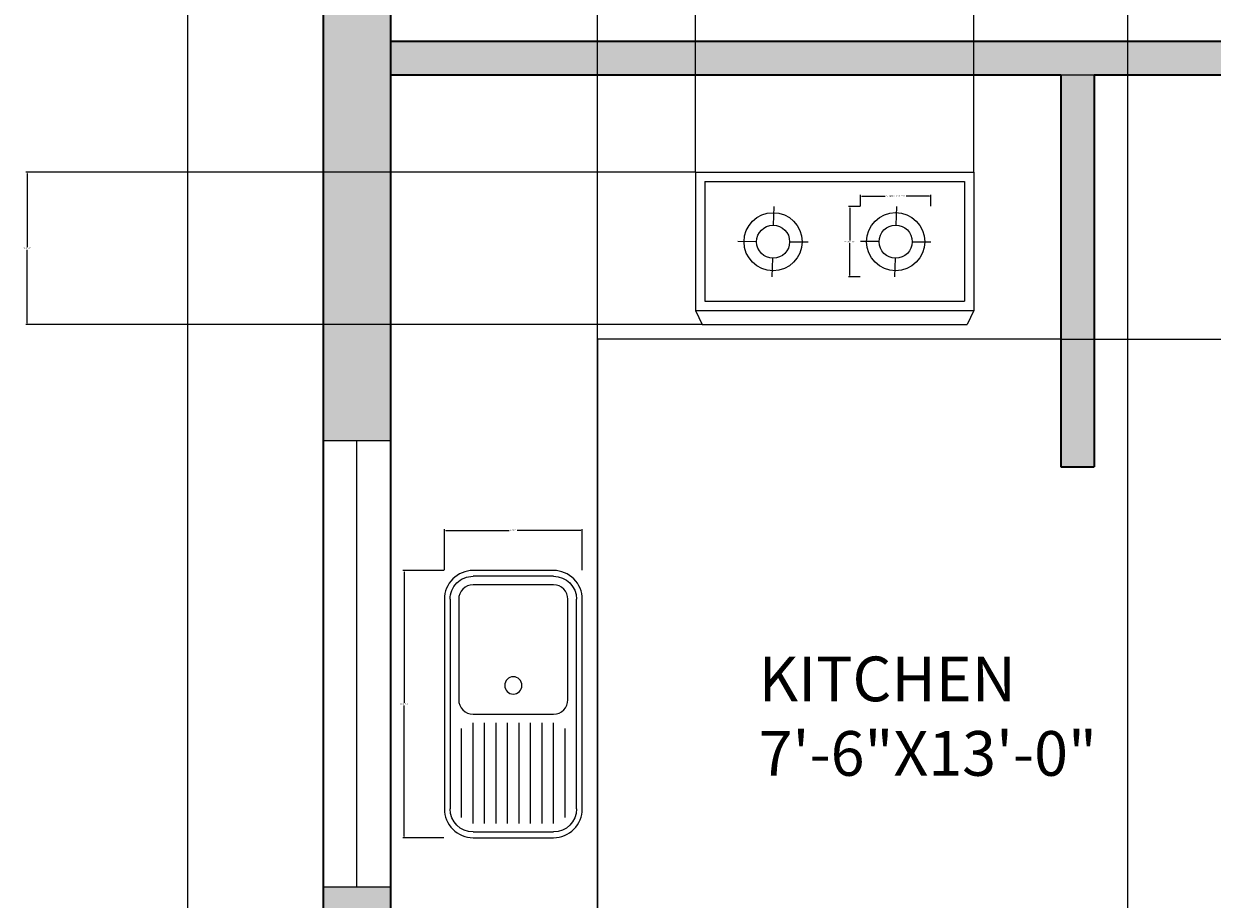
# Model space of a CAD drawing. Units: inches. Extents: x -15 to 423, y -713 to 71.
# Tile 2 of 24: x -15 to 144, y -351 to -234. Entities that reach past the tile are written whole.
import ezdxf

# ---------------------------------------------------------------- set-up
doc = ezdxf.new("R2010")
doc.units = ezdxf.units.IN
doc.header["$MEASUREMENT"] = 0
for name, color, linetype, lineweight in [('A-ANNO-DIMS', 2, 'Continuous', 18), ('A-AREA-IDEN', 7, 'Continuous', 18), ('A-FLOR-CASE', 7, 'Continuous', 25), ('A-GLAZ', 5, 'Continuous', 18), ('A-WALL', 7, 'Continuous', 35), ('A-WALL-PATT', 8, 'Continuous', 13), ('equipments', 7, 'Continuous', 18)]:
    doc.layers.add(name, color=color, linetype=linetype, lineweight=lineweight)
doc.styles.get("Standard").update_dxf_attribs({"font": 'arial.ttf'})
doc.dimstyles.get("Standard").update_dxf_attribs({"dimtxt": 0.18, "dimasz": 0.18, "dimexe": 0.18, "dimexo": 0.0625, "dimgap": 0.09, "dimtad": 0, "dimtih": 1, "dimtoh": 1, "dimdec": 0, "dimzin": 0, "dimdsep": 46, "dimlunit": 3, "dimtxsty": 'Standard', "dimcen": 0.09, "dimadec": 0, "dimazin": 0, "dimtfac": 1, "dimtdec": 0, "dimtofl": 0, "dimtmove": 0, "dimatfit": 3, "dimfxl": 1, "dimtolj": 1, "dimtzin": 0, "dimarcsym": 0})

# ---------------------------------------------------------------- blocks, each defined once
blk = doc.blocks.new('SINK_KITCHEN_SNGL')
for p, q in [((-36.5, -2), (36.5, -2)), ((-39.5, -6), (-8.5, -6)), ((-44.5, -38), (-44.5, -10)), ((-41.5, -10), (-6.5, -10)), ((44.5, -10), (44.5, -38)), ((-41.5, -14), (-6.5, -14)), ((-41.5, -18), (-6.5, -18)), ((-41.5, -22), (-6.5, -22)), ((-41.5, -26), (-6.5, -26)), ((-41.5, -30), (-6.5, -30)), ((-41.5, -34), (-6.5, -34)), ((-41.5, -38), (-6.5, -38)), ((-39.5, -42), (-8.5, -42)), ((36.5, -46), (-36.5, -46))]:
    blk.add_line(p, q)
at = {"flags": 128}
for points in [[(36.5, 0, -0.414214), (46.5, -10), (46.5, -38, -0.414214), (36.5, -48), (-36.5, -48, -0.414214), (-46.5, -38), (-46.5, -10, -0.414214), (-36.5, 0)], [(36.5, -5, -0.414214), (41.5, -10), (41.5, -38, -0.414214), (36.5, -43), (1.5, -43, -0.414214), (-3.5, -38), (-3.5, -10, -0.414214), (1.5, -5)]]:
    blk.add_lwpolyline(points, format="xyb", close=True, dxfattribs=at)
blk.add_circle((6.5, -24), 3)
for centre, start, end in [((-36.5, -10), 90, 180), ((36.5, -10), 0, 90), ((-36.5, -38), 180, 270), ((36.5, -38), 270, 0)]:
    blk.add_arc(centre, 8, start, end)
blk = doc.blocks.new('*D8')
at = {"layer": 'A-ANNO-DIMS', "color": 0, "lineweight": -2, "transparency": 16777216}
for p, q in [((25.02, 17.5), (6.72, 17.5)), ((6.9, 17.32), (6.9, -193.09)), ((6.9, -409.82), (6.9, -199.41)), ((34.02, -410), (6.72, -410))]:
    blk.add_line(p, q, dxfattribs=at)
at = {"layer": 'A-ANNO-DIMS', "color": 0, "transparency": 16777216}
for points in [[(6.87, 17.32), (6.93, 17.32), (6.9, 17.5)], [(6.87, -409.82), (6.93, -409.82), (6.9, -410)]]:
    blk.add_solid(points, dxfattribs=at)
at = {"layer": 'Defpoints', "color": 0, "transparency": 16777216}
for p in [(25.08, 17.5), (6.9, -410), (34.08, -410)]:
    blk.add_point(p, dxfattribs=at)
at = {"layer": 'A-ANNO-DIMS', "color": 0, "transparency": 16777216, "insert": (6.9, -196.25), "char_height": 6, "attachment_point": 5}
blk.add_mtext('\\A1;35\'-8"', dxfattribs=at)
blk = doc.blocks.new('WINDOW-60IN')
for p, q in [((0, 9), (60, 9)), ((0, 0), (0, 9)), ((60, 9), (60, 0)), ((0, 4.5), (60, 4.5)), ((60, 0), (0, 0))]:
    blk.add_line(p, q)
blk = doc.blocks.new('COOKTOP-BURNER')
for p, q in [((4.78, 6.93), (4.86, 9.43)), ((2.5, 4.72), (0, 4.74)), ((6.94, 4.7), (9.43, 4.69)), ((4.65, 2.49), (4.57, 0))]:
    blk.add_line(p, q)
for radius in [3.9, 2.22]:
    blk.add_circle((4.72, 4.71), radius)
blk = doc.blocks.new('*D33')
at = {"layer": 'A-ANNO-DIMS', "color": 0, "lineweight": -2, "transparency": 16777216}
for p, q in [((97.2, -258.14), (97.2, -256.61)), ((97.38, -256.79), (100.5, -256.79)), ((106.45, -256.79), (103.32, -256.79)), ((106.63, -258.14), (106.63, -256.61))]:
    blk.add_line(p, q, dxfattribs=at)
at = {"layer": 'A-ANNO-DIMS', "color": 0, "transparency": 16777216}
for points in [[(97.38, -256.76), (97.38, -256.82), (97.2, -256.79)], [(106.45, -256.76), (106.45, -256.82), (106.63, -256.79)]]:
    blk.add_solid(points, dxfattribs=at)
at = {"layer": 'Defpoints', "color": 0, "transparency": 16777216}
for p in [(97.2, -256.79), (97.2, -258.2), (106.63, -258.2)]:
    blk.add_point(p, dxfattribs=at)
at = {"layer": 'A-ANNO-DIMS', "color": 0, "transparency": 16777216, "insert": (101.91, -256.79), "char_height": 0.18, "attachment_point": 5}
blk.add_mtext('\\A1;BURNER 0\'-9 1/2" TYP.', dxfattribs=at)
blk = doc.blocks.new('*D34')
at = {"layer": 'A-ANNO-DIMS', "color": 0, "lineweight": -2, "transparency": 16777216}
for p, q in [((97.14, -258.2), (95.6, -258.2)), ((95.78, -258.38), (95.78, -262.73)), ((95.78, -267.45), (95.78, -263.1)), ((97.14, -267.63), (95.6, -267.63))]:
    blk.add_line(p, q, dxfattribs=at)
at = {"layer": 'A-ANNO-DIMS', "color": 0, "transparency": 16777216}
for points in [[(95.75, -258.38), (95.81, -258.38), (95.78, -258.2)], [(95.75, -267.45), (95.81, -267.45), (95.78, -267.63)]]:
    blk.add_solid(points, dxfattribs=at)
at = {"layer": 'Defpoints', "color": 0, "transparency": 16777216}
for p in [(97.2, -258.2), (95.78, -267.63), (97.2, -267.63)]:
    blk.add_point(p, dxfattribs=at)
at = {"layer": 'A-ANNO-DIMS', "color": 0, "transparency": 16777216, "insert": (95.78, -262.91), "char_height": 0.18, "attachment_point": 5}
blk.add_mtext('\\A1;0\'-9 1/2" TYP.', dxfattribs=at)
blk = doc.blocks.new('*D35')
at = {"layer": 'A-ANNO-DIMS', "color": 0, "lineweight": -2, "transparency": 16777216}
for p, q in [((41.26, -307.05), (35.77, -307.05)), ((35.95, -307.23), (35.95, -324.81)), ((35.95, -342.75), (35.95, -325.17)), ((41.26, -342.93), (35.77, -342.93))]:
    blk.add_line(p, q, dxfattribs=at)
at = {"layer": 'A-ANNO-DIMS', "color": 0, "transparency": 16777216}
for points in [[(35.92, -307.23), (35.98, -307.23), (35.95, -307.05)], [(35.92, -342.75), (35.98, -342.75), (35.95, -342.93)]]:
    blk.add_solid(points, dxfattribs=at)
at = {"layer": 'Defpoints', "color": 0, "transparency": 16777216}
for p in [(35.95, -307.05), (41.33, -307.05), (41.33, -342.93)]:
    blk.add_point(p, dxfattribs=at)
at = {"layer": 'A-ANNO-DIMS', "color": 0, "transparency": 16777216, "insert": (35.95, -324.99), "char_height": 0.18, "attachment_point": 5}
blk.add_mtext('\\A1;SINK 3\'-0"', dxfattribs=at)
blk = doc.blocks.new('*D36')
at = {"layer": 'A-ANNO-DIMS', "color": 0, "lineweight": -2, "transparency": 16777216}
for p, q in [((41.33, -306.99), (41.33, -301.49)), ((59.84, -306.99), (59.84, -301.49)), ((41.51, -301.67), (50.05, -301.67)), ((59.66, -301.67), (51.11, -301.67))]:
    blk.add_line(p, q, dxfattribs=at)
at = {"layer": 'A-ANNO-DIMS', "color": 0, "transparency": 16777216}
for points in [[(41.51, -301.64), (41.51, -301.7), (41.33, -301.67)], [(59.66, -301.64), (59.66, -301.7), (59.84, -301.67)]]:
    blk.add_solid(points, dxfattribs=at)
at = {"layer": 'Defpoints', "color": 0, "transparency": 16777216}
for p in [(59.84, -301.67), (41.33, -307.05), (59.84, -307.05)]:
    blk.add_point(p, dxfattribs=at)
at = {"layer": 'A-ANNO-DIMS', "color": 0, "transparency": 16777216, "insert": (50.58, -301.67), "char_height": 0.18, "attachment_point": 5}
blk.add_mtext('\\A1;1\'-6 1/2"', dxfattribs=at)
blk = doc.blocks.new('*D37')
at = {"layer": 'A-ANNO-DIMS', "color": 0, "lineweight": -2, "transparency": 16777216}
for p, q in [((34.08, -396.44), (34.08, 57.43)), ((34.26, 57.25), (47.65, 57.25)), ((61.7, 57.25), (48.31, 57.25)), ((61.88, -396.44), (61.88, 57.43))]:
    blk.add_line(p, q, dxfattribs=at)
at = {"layer": 'A-ANNO-DIMS', "color": 0, "transparency": 16777216}
for points in [[(34.26, 57.28), (34.26, 57.22), (34.08, 57.25)], [(61.7, 57.28), (61.7, 57.22), (61.88, 57.25)]]:
    blk.add_solid(points, dxfattribs=at)
at = {"layer": 'Defpoints', "color": 0, "transparency": 16777216}
for p in [(61.88, 57.25), (34.08, -396.5), (61.88, -396.5)]:
    blk.add_point(p, dxfattribs=at)
at = {"layer": 'A-ANNO-DIMS', "color": 0, "transparency": 16777216, "insert": (47.98, 57.25), "char_height": 0.18, "attachment_point": 5}
blk.add_mtext('\\A1;2\'-4"', dxfattribs=at)
blk = doc.blocks.new('*D38')
at = {"layer": 'A-ANNO-DIMS', "color": 0, "lineweight": -2, "transparency": 16777216}
for p, q in [((124.14, -240.5), (422.01, -240.5)), ((421.83, -240.68), (421.83, -258.06)), ((421.83, -275.8), (421.83, -258.42)), ((124.14, -275.98), (422.01, -275.98))]:
    blk.add_line(p, q, dxfattribs=at)
at = {"layer": 'A-ANNO-DIMS', "color": 0, "transparency": 16777216}
for points in [[(421.8, -240.68), (421.86, -240.68), (421.83, -240.5)], [(421.8, -275.8), (421.86, -275.8), (421.83, -275.98)]]:
    blk.add_solid(points, dxfattribs=at)
at = {"layer": 'Defpoints', "color": 0, "transparency": 16777216}
for p in [(124.08, -240.5), (124.08, -275.98), (421.83, -275.98)]:
    blk.add_point(p, dxfattribs=at)
at = {"layer": 'A-ANNO-DIMS', "color": 0, "transparency": 16777216, "insert": (421.83, -258.24), "char_height": 0.18, "attachment_point": 5}
blk.add_mtext('\\A1;2\'-11 1/2"', dxfattribs=at)
blk = doc.blocks.new('*D39')
at = {"layer": 'A-ANNO-DIMS', "color": 0, "lineweight": -2, "transparency": 16777216}
for p, q in [((75.05, -253.53), (75.05, 57.43)), ((75.23, 57.25), (93.19, 57.25)), ((112.22, 57.25), (94.26, 57.25)), ((112.4, -253.53), (112.4, 57.43))]:
    blk.add_line(p, q, dxfattribs=at)
at = {"layer": 'A-ANNO-DIMS', "color": 0, "transparency": 16777216}
for points in [[(75.23, 57.28), (75.23, 57.22), (75.05, 57.25)], [(112.22, 57.28), (112.22, 57.22), (112.4, 57.25)]]:
    blk.add_solid(points, dxfattribs=at)
at = {"layer": 'Defpoints', "color": 0, "transparency": 16777216}
for p in [(112.4, 57.25), (75.05, -253.59), (112.4, -253.59)]:
    blk.add_point(p, dxfattribs=at)
at = {"layer": 'A-ANNO-DIMS', "color": 0, "transparency": 16777216, "insert": (93.72, 57.25), "char_height": 0.18, "attachment_point": 5}
blk.add_mtext('\\A1;3\'-1 1/2"', dxfattribs=at)
blk = doc.blocks.new('*D40')
at = {"layer": 'A-ANNO-DIMS', "color": 0, "lineweight": -2, "transparency": 16777216}
for p, q in [((74.99, -253.59), (-14.85, -253.59)), ((-14.67, -253.77), (-14.67, -263.63)), ((-14.67, -273.85), (-14.67, -263.99)), ((75.86, -274.03), (-14.85, -274.03))]:
    blk.add_line(p, q, dxfattribs=at)
at = {"layer": 'A-ANNO-DIMS', "color": 0, "transparency": 16777216}
for points in [[(-14.7, -253.77), (-14.64, -253.77), (-14.67, -253.59)], [(-14.7, -273.85), (-14.64, -273.85), (-14.67, -274.03)]]:
    blk.add_solid(points, dxfattribs=at)
at = {"layer": 'Defpoints', "color": 0, "transparency": 16777216}
for p in [(75.05, -253.59), (-14.67, -274.03), (75.92, -274.03)]:
    blk.add_point(p, dxfattribs=at)
at = {"layer": 'A-ANNO-DIMS', "color": 0, "transparency": 16777216, "insert": (-14.67, -263.81), "char_height": 0.18, "attachment_point": 5}
blk.add_mtext('\\A1;1\'-8 1/2"', dxfattribs=at)
blk = doc.blocks.new('*D42')
at = {"layer": 'A-ANNO-DIMS', "color": 0, "lineweight": -2, "transparency": 16777216}
for p, q in [((133.08, -409.94), (133.08, 57.43)), ((133.26, 57.25), (157.25, 57.25)), ((181.9, 57.25), (157.91, 57.25)), ((182.08, -409.94), (182.08, 57.43))]:
    blk.add_line(p, q, dxfattribs=at)
at = {"layer": 'A-ANNO-DIMS', "color": 0, "transparency": 16777216}
for points in [[(133.26, 57.28), (133.26, 57.22), (133.08, 57.25)], [(181.9, 57.28), (181.9, 57.22), (182.08, 57.25)]]:
    blk.add_solid(points, dxfattribs=at)
at = {"layer": 'Defpoints', "color": 0, "transparency": 16777216}
for p in [(182.08, 57.25), (133.08, -410), (182.08, -410)]:
    blk.add_point(p, dxfattribs=at)
at = {"layer": 'A-ANNO-DIMS', "color": 0, "transparency": 16777216, "insert": (157.58, 57.25), "char_height": 0.18, "attachment_point": 5}
blk.add_mtext('\\A1;4\'-1"', dxfattribs=at)

msp = doc.modelspace()

# ---------------------------------------------------------------- hatches: boundary and pattern name
at = {"layer": 'A-WALL-PATT'}
h = msp.add_hatch(color=256, dxfattribs=at)
h.dxf.hatch_style = 1
h.paths.add_polyline_path([(34.08, -349.58), (25.08, -349.58), (25.08, -431), (34.08, -431)])
h.paths.add_polyline_path([(34.08, -467), (25.08, -467), (25.08, -673), (34.08, -673)])
h.paths.add_polyline_path([(373.08, -668.5), (182.08, -668.5), (182.08, -673), (373.08, -673)])
h.paths.add_polyline_path([(253.2, -597.5), (191.08, -597.5), (191.08, -594.5), (182.08, -594.5), (182.08, -606.5), (253.2, -606.5)])
h.paths.add_polyline_path([(373.08, -597.5), (313.2, -597.5), (313.2, -606.5), (373.08, -606.5)])
h.paths.add_polyline_path([(382.08, -545.55), (373.08, -545.55), (373.08, -673), (382.08, -673)])
h.paths.add_polyline_path([(139.08, -488), (34.08, -488), (34.08, -497), (139.08, -497), (139.08, -492.5)])
h.paths.add_polyline_path([(139.08, -396.5), (128.58, -396.5), (128.58, -352.79), (124.08, -352.79), (124.08, -396.5), (34.08, -396.5), (34.08, -410), (139.08, -410), (139.08, -403.25)])
h.paths.add_polyline_path([(191.08, -396.5), (179.08, -396.5), (179.08, -410), (182.08, -410), (182.08, -488), (179.08, -488), (179.08, -497), (182.08, -497), (182.08, -501.43), (191.08, -501.43)])
h.paths.add_polyline_path([(373.08, -396.5), (253.08, -396.5), (253.08, -393.5), (248.58, -393.5), (248.58, -401), (284.58, -401), (284.58, -404), (289.08, -404), (289.08, -401), (373.08, -401)])
h.paths.add_polyline_path([(373.08, -449), (289.08, -449), (289.08, -432), (286.83, -432), (284.58, -432), (284.58, -453.5), (373.08, -453.5)])
h.paths.add_polyline_path([(382.08, -344.27), (373.08, -344.27), (373.08, -413.68), (382.08, -413.68)])
h.paths.add_polyline_path([(382.08, -437.68), (373.08, -437.68), (373.08, -485.55), (382.08, -485.55)])
h.paths.add_polyline_path([(34.08, -188.26), (25.08, -188.26), (25.08, -289.58), (34.08, -289.58)])
h.paths.add_polyline_path([(164.08, -236), (34.08, -236), (34.08, -240.5), (124.08, -240.5), (124.08, -293.12), (128.58, -293.12), (128.58, -240.5), (164.08, -240.5), (164.08, -238.25)])
h.paths.add_polyline_path([(373.08, -236), (242.58, -236), (242.58, -238.25), (242.58, -240.5), (248.58, -240.5), (248.58, -353.5), (250.83, -353.5), (253.08, -353.5), (253.08, -240.5), (373.08, -240.5)])
h.paths.add_polyline_path([(382.08, -190.86), (373.08, -190.86), (373.08, -284.27), (382.08, -284.27)])
h.paths.add_polyline_path([(211.58, -80), (253.58, -80), (253.58, -77.75), (253.58, -75.5), (153.58, -75.5), (153.58, -77.75), (153.58, -80), (207.08, -80), (207.08, -236), (204.08, -236), (204.08, -240.5), (214.58, -240.5), (214.58, -236), (211.58, -236)])
h.paths.add_polyline_path([(34.08, 8.5), (70.36, 8.5), (70.36, 17.5), (25.08, 17.5), (25.08, -128.26), (34.08, -128.26)])
h.paths.add_polyline_path([(110.58, 17.5), (94.36, 17.5), (94.36, 8.5), (110.58, 8.5)])
h.paths.add_polyline_path([(296.58, 17.5), (110.58, 17.5), (110.58, 13), (296.58, 13)])
h.paths.add_polyline_path([(110.58, 8.5), (106.08, 8.5), (106.08, -75.5), (103.08, -75.5), (103.08, -80), (113.58, -80), (113.58, -77.75), (113.58, -75.5), (110.58, -75.5)])
h.paths.add_polyline_path([(75.08, -75.5), (34.08, -75.5), (34.08, -80), (75.08, -80), (75.08, -77.75)])
h.paths.add_polyline_path([(343.09, 17.5), (296.58, 17.5), (296.58, 13), (296.58, 8.5), (343.09, 8.5)])
h.paths.add_polyline_path([(304.08, -75.5), (301.08, -75.5), (301.08, 8.5), (296.58, 8.5), (296.58, -75.5), (293.58, -75.5), (293.58, -80), (304.08, -80)])
h.paths.add_polyline_path([(382.08, 17.5), (367.09, 17.5), (367.09, 8.5), (373.08, 8.5), (373.08, -130.86), (382.08, -130.86)])
h.paths.add_polyline_path([(373.08, -75.5), (332.08, -75.5), (332.08, -77.75), (332.08, -80), (373.08, -80)])

# ---------------------------------------------------------------- linework, layer by layer
at = {"layer": 'A-FLOR-CASE'}
for p, q in [((124.08, -275.98), (61.88, -275.98)), ((61.88, -275.98), (61.88, -396.5))]:
    msp.add_line(p, q, dxfattribs=at)
at = {"layer": 'A-WALL'}
for p, q in [((25.08, 17.5), (25.08, -673)), ((34.08, 8.5), (34.08, -673)), ((34.08, -236), (164.08, -236)), ((34.08, -240.5), (124.08, -240.5)), ((124.08, -240.5), (124.08, -293.12)), ((128.58, -240.5), (128.58, -293.12)), ((128.58, -240.5), (248.58, -240.5)), ((124.08, -293.12), (128.58, -293.12))]:
    msp.add_line(p, q, dxfattribs=at)
at = {"layer": 'equipments'}
for p, q in [((75.05, -253.59), (75.05, -272.14)), ((75.05, -253.59), (112.4, -253.59)), ((112.4, -253.59), (112.4, -272.14)), ((76.3, -254.84), (76.3, -270.89)), ((76.3, -254.84), (111.15, -254.84)), ((111.15, -254.84), (111.15, -270.89)), ((76.3, -270.89), (111.15, -270.89)), ((75.05, -272.14), (112.4, -272.14)), ((75.05, -272.14), (75.92, -274.03)), ((112.4, -272.14), (111.53, -274.03)), ((75.92, -274.03), (111.53, -274.03))]:
    msp.add_line(p, q, dxfattribs=at)

# ---------------------------------------------------------------- block references
at = {"layer": 'A-GLAZ', "rotation": 89.99999999999996}
msp.add_blockref('WINDOW-60IN', (34.08, -349.58), dxfattribs=at)
at = {"layer": 'equipments'}
msp.add_blockref('COOKTOP-BURNER', (80.74, -267.63), dxfattribs=at)
at = {"layer": 'equipments', "rotation": 180}
msp.add_blockref('COOKTOP-BURNER', (106.63, -258.2), dxfattribs=at)
at = {"layer": 'equipments', "xscale": -0.3857018310003651, "yscale": 0.3857018310003651, "zscale": 0.3857018310003651, "rotation": 270}
msp.add_blockref('SINK_KITCHEN_SNGL', (59.84, -324.99), dxfattribs=at)

# ---------------------------------------------------------------- texts
at = {"layer": 'A-AREA-IDEN', "insert": (83.53, -318.61), "char_height": 6, "attachment_point": 1}
msp.add_mtext('KITCHEN\\P7\'-6"X13\'-0"', dxfattribs=at)

# ---------------------------------------------------------------- dimensions: what is measured, and where the dimension line sits
at = {"layer": 'A-ANNO-DIMS'}
for base, p1, p2, picture, middle in [((112.3972, 57.2501), (75.0509, -253.5887), (112.3972, -253.5887), '*D39', (93.724, 57.2501)), ((61.88, 57.25), (34.08, -396.5), (61.88, -396.5), '*D37', (47.98, 57.25)), ((182.08, 57.25), (133.08, -410), (182.08, -410), '*D42', (157.58, 57.25)), ((59.84, -301.67), (41.33, -307.05), (59.84, -307.05), '*D36', (50.58, -301.67))]:
    dim = msp.add_linear_dim(base=base, p1=p1, p2=p2, dimstyle='Standard', override={"dimdec": 1, "dimlfac": 1, "dimrnd": 0, "dimzin": 1, "dimdsep": 46, "dimlunit": 4, "dimfrac": 2}, dxfattribs=at)
    dim.commit()
    dim.dimension.update_dxf_attribs({"geometry": picture, "text_midpoint": middle})
for base, p1, p2, override, picture, middle in [((6.9041327, -409.99989936), (25.08055573, 17.50010064), (34.08055573, -409.99989936), {"dimtxt": 6, "dimclrd": 0, "dimclre": 0, "dimclrt": 0}, '*D8', (6.9041327, -196.24989936)), ((421.83, -275.98), (124.08, -240.5), (124.08, -275.98), {"dimdec": 1, "dimlfac": 1, "dimrnd": 0, "dimzin": 1, "dimdsep": 46, "dimlunit": 4, "dimfrac": 2}, '*D38', (421.83, -258.24)), ((-14.67, -274.03), (75.05, -253.59), (75.92, -274.03), {"dimdec": 1, "dimlfac": 1, "dimrnd": 0, "dimzin": 1, "dimdsep": 46, "dimlunit": 4, "dimfrac": 2}, '*D40', (-14.67, -263.81))]:
    dim = msp.add_linear_dim(base=base, p1=p1, p2=p2, angle=90, dimstyle='Standard', override=override, dxfattribs=at)
    dim.commit()
    dim.dimension.update_dxf_attribs({"geometry": picture, "text_midpoint": middle})
for base, p1, p2, angle, text, picture, middle in [((97.2, -256.79), (106.63, -258.2), (97.2, -258.2), 180, 'BURNER <> TYP.', '*D33', (101.91, -256.79)), ((95.78, -267.63), (97.2, -258.2), (97.2, -267.63), 270, '<> TYP.', '*D34', (95.78, -262.91)), ((35.95, -307.05), (41.33, -342.93), (41.33, -307.05), 90, 'SINK <>', '*D35', (35.95, -324.99))]:
    dim = msp.add_linear_dim(base=base, p1=p1, p2=p2, angle=angle, text=text, dimstyle='Standard', override={"dimdec": 1, "dimlfac": 1, "dimrnd": 0, "dimzin": 1, "dimdsep": 46, "dimlunit": 4, "dimfrac": 2}, dxfattribs=at)
    dim.commit()
    dim.dimension.update_dxf_attribs({"geometry": picture, "text_midpoint": middle})

doc.saveas('drawing.dxf')
